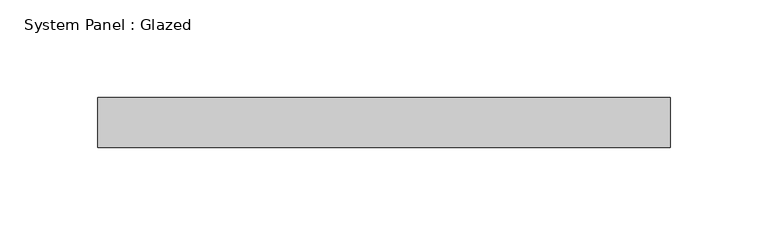
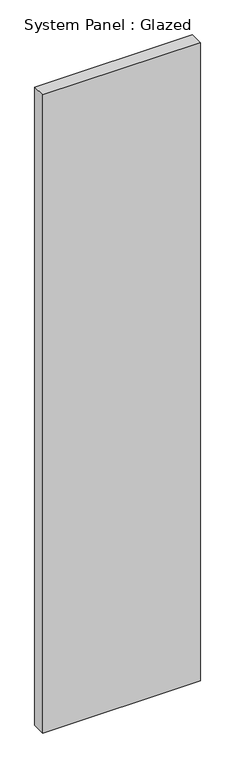
"""IFC4 building model written with IfcOpenShell, lengths in millimetres: plate geometry, System Panel : Glazed."""

from ifc_helpers import new_model, si_unit, origin, origin_with_axes, place, context, project, spatial, polyline, outline, extrude, source, transform, mapped, element, save


def system_panel_glazed_199a1f6c(model_context):
    return source(origin(), model_context, "Body", "SweptSolid", [
        extrude(outline(polyline([(146.05, 19.05), (-146.05, 19.05), (-146.05, 44.45), (146.05, 44.45), (146.05, 19.05)])), origin_with_axes(), (0.0, 0.0, 1.0), 1249.6336497),
    ])


if __name__ == "__main__":
    model = new_model("IFC4")
    model_context = context("Model", 3, world=origin())
    ifc_project = project(units=[si_unit("LENGTHUNIT", "METRE", prefix="MILLI")], contexts=[model_context])
    site = spatial("IfcSite", under=ifc_project)
    building = spatial("IfcBuilding", under=site)
    placement = place(None, origin())
    system_panel_glazed_shape = system_panel_glazed_199a1f6c(model_context)
    element("IfcPlate", 1, ObjectType="System Panel : Glazed", at=placement, inside=building, context=model_context, shape_type="MappedRepresentation", body=[
        mapped(system_panel_glazed_shape, transform((0.0, 0.0, 0.0), x_axis=(1.0, 0.0, 0.0), y_axis=(0.0, 1.0, 0.0), z_axis=(0.0, 0.0, 1.0))),
    ])
    save(model, "model.ifc")

# Revit data of these elements
# Type "System Panel : Glazed"
#   Construction Type Id = "GSP4R"
#   Analytic Construction = "1/8 in Pilkington single glazing"
#   Visual Light Transmittance = 0.9
#   Solar Heat Gain Coefficient = 0.86
#   Heat Transfer Coefficient (U) = 1.18115 BTU/(h·ft²·°F)
#   Define Thermal Properties by = 1
# Element 1 (IfcPlate, "System Panel : Glazed")
#   Materials on its faces: "Glass"
# Materials
#   "Glass": class "Glass", colour RGB 0 128 192, transparency 0.75, Description = "Soda Lime Glass", Cost = 0
